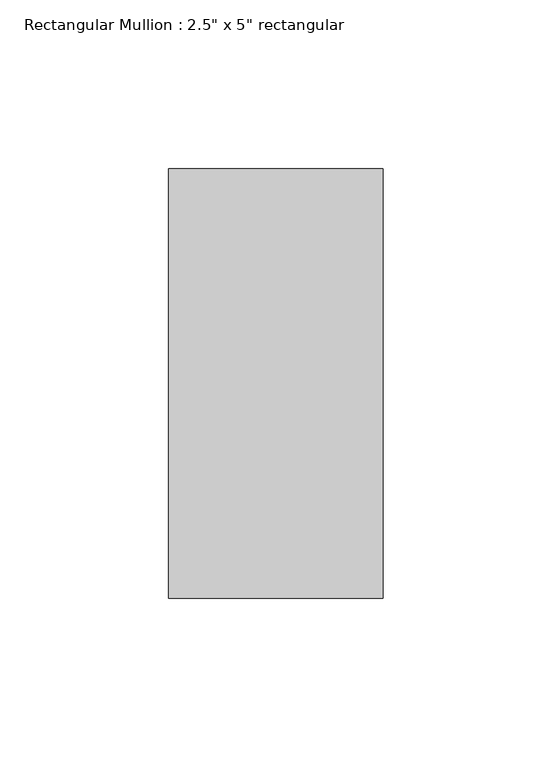
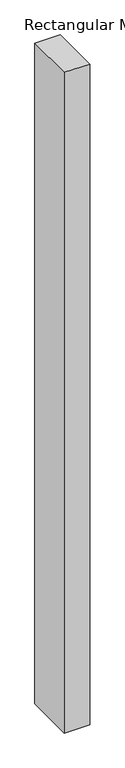
"""IFC4 building model written with IfcOpenShell, lengths in millimetres: member geometry."""

from ifc_helpers import new_model, si_unit, frame, origin, place, context, project, spatial, polyline, outline, extrude, source, transform, mapped, element, save


def member_d8304dce(model_context):
    return source(origin(), model_context, "Body", "SweptSolid", [
        extrude(outline(polyline([(31.75, 63.5), (31.75, -63.5), (-31.75, -63.5), (-31.75, 63.5), (31.75, 63.5)])), frame((0.0, 0.0, -1744.0799136), z_axis=(0.0, 0.0, 1.0), x_axis=(1.0, 0.0, 0.0)), (0.0, 0.0, 1.0), 1744.0799136),
    ])


if __name__ == "__main__":
    model = new_model("IFC4")
    model_context = context("Model", 3, world=origin())
    ifc_project = project(units=[si_unit("LENGTHUNIT", "METRE", prefix="MILLI")], contexts=[model_context])
    site = spatial("IfcSite", under=ifc_project)
    building = spatial("IfcBuilding", under=site)
    placement = place(None, origin())
    member_shape = member_d8304dce(model_context)
    element("IfcMember", 1, ObjectType="Rectangular Mullion : 2.5\" x 5\" rectangular", at=placement, inside=building, context=model_context, shape_type="MappedRepresentation", body=[
        mapped(member_shape, transform((0.0, 0.0, 0.0), x_axis=(1.0, 0.0, 0.0), y_axis=(0.0, 1.0, 0.0), z_axis=(0.0, 0.0, 1.0))),
    ])
    save(model, "model.ifc")

# Revit data of these elements
# Type "Rectangular Mullion : 2.5\" x 5\" rectangular"
#   built-in parameter 1007304 = 0.416667 (stored number, unit not read)
#   built-in parameter 1007301 = 0.104167 (stored number, unit not read)
#   built-in parameter 1007300 = 0.104167 (stored number, unit not read)
# Element 1 (IfcMember, "Rectangular Mullion : 2.5\" x 5\" rectangular")
#   Materials on its faces: "Aluminum"
# Materials
#   "Aluminum": class "Metal", colour RGB 247 247 247, transparency 0, Description = "Aluminum 6061", Cost = 0
